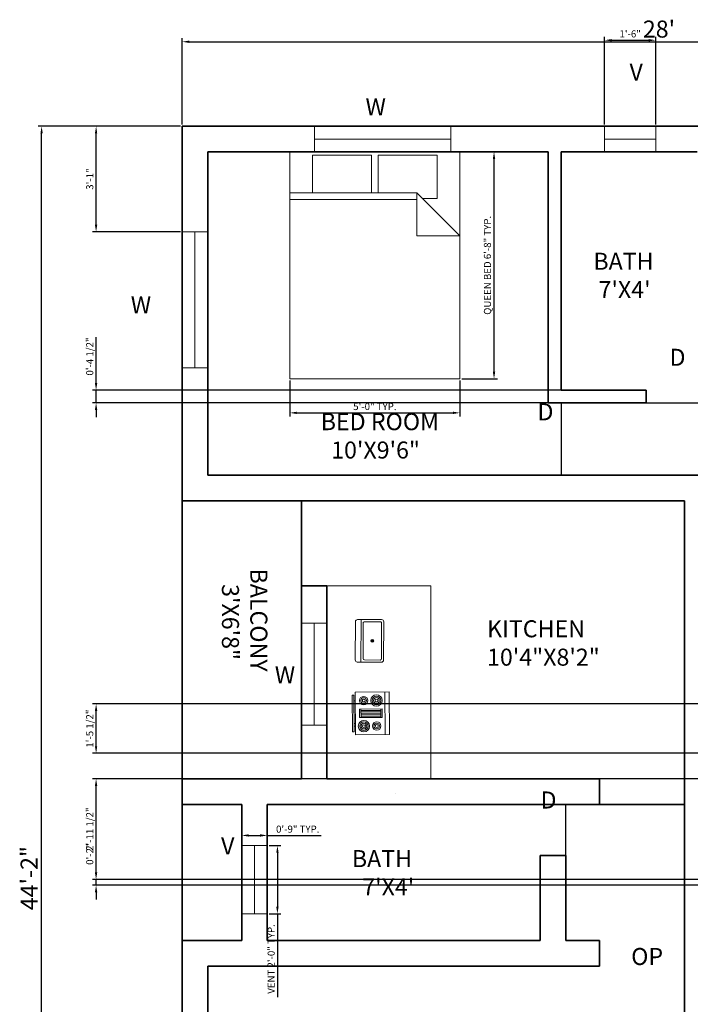
# Model space of a CAD drawing. Units: inches. Extents: x 22580 to 27643822, y 20781 to 31007121.
# Tile 2 of 3: x 27643397 to 27643633, y 31006774 to 31007121. Entities that reach past the tile are written whole.
import ezdxf

# ---------------------------------------------------------------- set-up
doc = ezdxf.new("R2010")
doc.units = ezdxf.units.IN
for name, color, linetype, lineweight in [('A-ANNO-DIMS', 2, 'Continuous', 18), ('A-ANNO-TEXT', 7, 'Continuous', 18), ('A-AREA-IDEN', 7, 'Continuous', 25), ('A-DOOR', 3, 'Continuous', 25), ('A-EQPM', 8, 'Continuous', 18), ('A-FLOR-CASE', 8, 'Continuous', 20), ('A-FLOR-FIXT', 9, 'Continuous', 18), ('A-FURN', 8, 'Continuous', 18), ('A-GLAZ', 4, 'Continuous', 18), ('A-REFR', 8, 'Continuous', 13), ('A-WALL', 7, 'Continuous', 35)]:
    doc.layers.add(name, color=color, linetype=linetype, lineweight=lineweight)
doc.styles.get("Standard").update_dxf_attribs({"font": 'arial.ttf'})
doc.dimstyles.new('ISO-25', dxfattribs={"dimtxt": 2.5, "dimasz": 2.5, "dimexe": 1.25, "dimexo": 0.625, "dimtad": 1, "dimdec": 1, "dimlunit": 3, "dimtxsty": 'Standard', "dimcen": 2.5, "dimadec": 0, "dimazin": 0, "dimtfac": 1, "dimtdec": 1, "dimtmove": 0, "dimatfit": 3, "dimfxl": 1, "dimarcsym": 0})

# ---------------------------------------------------------------- blocks, each defined once
blk = doc.blocks.new('Range-Oven - 30 in top')
for p, q in [((0, -3), (30, -3)), ((12, -6), (18, -6)), ((13, -20), (13, -6)), ((14, -6), (14, -20)), ((15, -20), (15, -6)), ((16, -6), (16, -20)), ((17, -20), (17, -6)), ((18, -20), (12, -20)), ((6, -24), (6, -25)), ((8, -25), (8, -24)), ((22, -25), (22, -24)), ((24, -24), (24, -25))]:
    blk.add_line(p, q)
for points in [[(0, -24), (0, 0), (30, 0), (30, -24)], [(12, -21), (12, -5), (18, -5), (18, -21)], [(2, -26), (2, -25), (28, -25), (28, -26)]]:
    blk.add_lwpolyline(points, close=True)
for centre, radius in [((6, -9), 4), ((6, -9), 3), ((24, -9), 3), ((6, -9), 2), ((6, -9), 1), ((24, -9), 2), ((24, -9), 1), ((6, -18), 3), ((6, -18), 2), ((6, -18), 1), ((24, -18), 4), ((24, -18), 3), ((24, -18), 2), ((24, -18), 1)]:
    blk.add_circle(centre, radius)
blk = doc.blocks.new('Bed - Queen')
for p, q in [((0, -80.00003), (0, 0)), ((0, 0), (59.99999, 0)), ((59.99999, 0), (59.99999, -80.00003)), ((7.99999, -1.2), (28.79998, -1.2)), ((7.99999, -14.4), (7.99999, -1.2)), ((28.79998, -1.2), (28.79998, -14.4)), ((31.19999, -1.2), (51.99999, -1.2)), ((31.19999, -14.4), (31.19999, -1.2)), ((51.99999, -1.2), (51.99999, -16.4)), ((0, -14.4), (44.8, -14.4)), ((44.8, -16.8), (0, -16.8)), ((59.99999, -29.6), (44.8, -14.4)), ((44.8, -14.4), (44.8, -29.6)), ((51.99999, -16.4), (46.79936, -16.4)), ((44.8, -29.6), (59.99999, -29.6)), ((59.99999, -80.00003), (0, -80.00003))]:
    blk.add_line(p, q)
blk = doc.blocks.new('Sink-single - 30 in top')
blk.add_line((-15, -3.999996), (15, -3.999996))
for points in [[(-13.5, 0), (13.5, 0)], [(-15, -18.499996), (-15, -1.5)], [(-13.5, -17.499996), (-13.5, -6.499996)], [(-12.5, -5.499996), (12.5, -5.499996)], [(13.5, -6.499996), (13.5, -17.499996)], [(15, -1.5), (15, -18.499996)], [(13.5, -19.999996), (-13.5, -19.999996)], [(12.5, -18.499996), (-12.5, -18.499996)]]:
    blk.add_lwpolyline(points)
for radius in [1, 0.5]:
    blk.add_circle((0, -11.999996), radius)
for centre, radius, start, end in [((-13.5, -1.5), 1.5, 90, 180), ((-12.5, -6.499996), 1, 90, 180), ((12.5, -6.499996), 1, 0, 90), ((13.5, -1.5), 1.5, 0, 90), ((-13.5, -18.499996), 1.5, 180, 270), ((-12.5, -17.499996), 1, 180, 270), ((12.5, -17.499996), 1, 270, 0), ((13.5, -18.499996), 1.5, 270, 0)]:
    blk.add_arc(centre, radius, start, end)
blk = doc.blocks.new('*D9')
at = {"layer": 'A-ANNO-DIMS', "color": 0, "lineweight": -2, "transparency": 16777216}
for p, q in [((27643453.96, 31007084.46), (27643453.96, 31007114.89)), ((27643456.46, 31007113.64), (27643787.46, 31007113.64)), ((27643789.96, 31007084.46), (27643789.96, 31007114.89))]:
    blk.add_line(p, q, dxfattribs=at)
at = {"layer": 'A-ANNO-DIMS', "color": 0, "transparency": 16777216}
for points in [[(27643456.46, 31007114.06), (27643456.46, 31007113.22), (27643453.96, 31007113.64)], [(27643787.46, 31007114.06), (27643787.46, 31007113.22), (27643789.96, 31007113.64)]]:
    blk.add_solid(points, dxfattribs=at)
at = {"layer": 'Defpoints', "color": 0, "transparency": 16777216}
for p in [(27643789.96, 31007113.64), (27643453.96, 31007083.83), (27643789.96, 31007083.83)]:
    blk.add_point(p, dxfattribs=at)
at = {"layer": 'A-ANNO-DIMS', "color": 0, "transparency": 16777216, "insert": (27643621.96, 31007117.33), "char_height": 6, "attachment_point": 5}
blk.add_mtext("28'", dxfattribs=at)
blk = doc.blocks.new('*D10')
at = {"layer": 'A-ANNO-DIMS', "color": 0, "lineweight": -2, "transparency": 16777216}
for p, q in [((27643453.33, 31007083.83), (27643403.16, 31007083.83)), ((27643404.41, 31006556.33), (27643404.41, 31007081.33)), ((27643453.33, 31006553.83), (27643403.16, 31006553.83))]:
    blk.add_line(p, q, dxfattribs=at)
at = {"layer": 'A-ANNO-DIMS', "color": 0, "transparency": 16777216}
for points in [[(27643404, 31007081.33), (27643404.83, 31007081.33), (27643404.41, 31007083.83)], [(27643404, 31006556.33), (27643404.83, 31006556.33), (27643404.41, 31006553.83)]]:
    blk.add_solid(points, dxfattribs=at)
at = {"layer": 'Defpoints', "color": 0, "transparency": 16777216}
for p in [(27643404.41, 31007083.83), (27643453.96, 31007083.83), (27643453.96, 31006553.83)]:
    blk.add_point(p, dxfattribs=at)
at = {"layer": 'A-ANNO-DIMS', "color": 0, "transparency": 16777216, "insert": (27643400.78, 31006818.83), "char_height": 6, "attachment_point": 5, "rotation": 90}
blk.add_mtext('44\'-2"', dxfattribs=at)
blk = doc.blocks.new('WIN-48IN')
for p, q in [((0, 9), (0, 0)), ((48, 9), (48, 0)), ((0, 4.5), (48, 4.5))]:
    blk.add_line(p, q)
blk = doc.blocks.new('VENT-24IN')
for p, q in [((0, 9), (0, 0)), ((24, 9), (24, 0)), ((0, 4.5), (24, 4.5))]:
    blk.add_line(p, q)
blk = doc.blocks.new('*D15')
at = {"layer": 'A-ANNO-DIMS', "color": 0, "lineweight": -2, "transparency": 16777216}
for p, q in [((27643484.54, 31006830.28), (27643488.76, 31006830.28)), ((27643487.51, 31006827.78), (27643487.51, 31006808.78)), ((27643484.54, 31006806.28), (27643488.76, 31006806.28)), ((27643487.51, 31006806.28), (27643487.51, 31006776.88))]:
    blk.add_line(p, q, dxfattribs=at)
at = {"layer": 'A-ANNO-DIMS', "color": 0, "transparency": 16777216}
for points in [[(27643487.09, 31006827.78), (27643487.93, 31006827.78), (27643487.51, 31006830.28)], [(27643487.09, 31006808.78), (27643487.93, 31006808.78), (27643487.51, 31006806.28)]]:
    blk.add_solid(points, dxfattribs=at)
at = {"layer": 'Defpoints', "color": 0, "transparency": 16777216}
for p in [(27643483.91, 31006830.28), (27643483.91, 31006806.28), (27643487.51, 31006806.28)]:
    blk.add_point(p, dxfattribs=at)
at = {"layer": 'A-ANNO-DIMS', "color": 0, "transparency": 16777216, "insert": (27643485.61, 31006790.33), "char_height": 2.5, "attachment_point": 5, "rotation": 90}
blk.add_mtext('VENT 2\'-0" TYP.', dxfattribs=at)
blk = doc.blocks.new('*D16')
at = {"layer": 'A-ANNO-DIMS', "color": 0, "lineweight": -2, "transparency": 16777216}
for p, q in [((27643474.91, 31006830.9), (27643474.91, 31006835.13)), ((27643483.91, 31006830.9), (27643483.91, 31006835.13)), ((27643477.41, 31006833.88), (27643481.41, 31006833.88)), ((27643483.91, 31006833.88), (27643502.9, 31006833.88))]:
    blk.add_line(p, q, dxfattribs=at)
at = {"layer": 'A-ANNO-DIMS', "color": 0, "transparency": 16777216}
for points in [[(27643477.41, 31006834.3), (27643477.41, 31006833.46), (27643474.91, 31006833.88)], [(27643481.41, 31006834.3), (27643481.41, 31006833.46), (27643483.91, 31006833.88)]]:
    blk.add_solid(points, dxfattribs=at)
at = {"layer": 'Defpoints', "color": 0, "transparency": 16777216}
for p in [(27643483.91, 31006833.88), (27643474.91, 31006830.28), (27643483.91, 31006830.28)]:
    blk.add_point(p, dxfattribs=at)
at = {"layer": 'A-ANNO-DIMS', "color": 0, "transparency": 16777216, "insert": (27643494.66, 31006835.78), "char_height": 2.5, "attachment_point": 5}
blk.add_mtext('0\'-9" TYP.', dxfattribs=at)
blk = doc.blocks.new('*D17')
at = {"layer": 'A-ANNO-DIMS', "color": 0, "lineweight": -2, "transparency": 16777216}
for p, q in [((27643552.46, 31007074.83), (27643565.09, 31007074.83)), ((27643563.84, 31006997.33), (27643563.84, 31007072.33)), ((27643552.46, 31006994.83), (27643565.09, 31006994.83))]:
    blk.add_line(p, q, dxfattribs=at)
at = {"layer": 'A-ANNO-DIMS', "color": 0, "transparency": 16777216}
for points in [[(27643563.42, 31007072.33), (27643564.25, 31007072.33), (27643563.84, 31007074.83)], [(27643563.42, 31006997.33), (27643564.25, 31006997.33), (27643563.84, 31006994.83)]]:
    blk.add_solid(points, dxfattribs=at)
at = {"layer": 'Defpoints', "color": 0, "transparency": 16777216}
for p in [(27643551.84, 31007074.83), (27643563.84, 31007074.83), (27643551.84, 31006994.83)]:
    blk.add_point(p, dxfattribs=at)
at = {"layer": 'A-ANNO-DIMS', "color": 0, "transparency": 16777216, "insert": (27643561.84, 31007034.83), "char_height": 2.5, "attachment_point": 5, "rotation": 90}
blk.add_mtext('QUEEN BED 6\'-8" TYP.', dxfattribs=at)
blk = doc.blocks.new('*D18')
at = {"layer": 'A-ANNO-DIMS', "color": 0, "lineweight": -2, "transparency": 16777216}
for p, q in [((27643491.84, 31006994.21), (27643491.84, 31006981.58)), ((27643551.84, 31006994.21), (27643551.84, 31006981.58)), ((27643494.34, 31006982.83), (27643549.34, 31006982.83))]:
    blk.add_line(p, q, dxfattribs=at)
at = {"layer": 'A-ANNO-DIMS', "color": 0, "transparency": 16777216}
for points in [[(27643494.34, 31006983.25), (27643494.34, 31006982.42), (27643491.84, 31006982.83)], [(27643549.34, 31006983.25), (27643549.34, 31006982.42), (27643551.84, 31006982.83)]]:
    blk.add_solid(points, dxfattribs=at)
at = {"layer": 'Defpoints', "color": 0, "transparency": 16777216}
for p in [(27643491.84, 31006994.83), (27643551.84, 31006994.83), (27643551.84, 31006982.83)]:
    blk.add_point(p, dxfattribs=at)
at = {"layer": 'A-ANNO-DIMS', "color": 0, "transparency": 16777216, "insert": (27643521.84, 31006984.74), "char_height": 2.5, "attachment_point": 5}
blk.add_mtext('5\'-0" TYP.', dxfattribs=at)
blk = doc.blocks.new('*D39')
at = {"layer": 'A-ANNO-DIMS', "color": 0, "lineweight": -2, "transparency": 16777216}
for p, q in [((27643661.33, 31006853.83), (27643422.36, 31006853.83)), ((27643423.61, 31006820.83), (27643423.61, 31006851.33)), ((27643661.33, 31006818.33), (27643422.36, 31006818.33))]:
    blk.add_line(p, q, dxfattribs=at)
at = {"layer": 'A-ANNO-DIMS', "color": 0, "transparency": 16777216}
for points in [[(27643423.19, 31006851.33), (27643424.02, 31006851.33), (27643423.61, 31006853.83)], [(27643423.19, 31006820.83), (27643424.02, 31006820.83), (27643423.61, 31006818.33)]]:
    blk.add_solid(points, dxfattribs=at)
at = {"layer": 'Defpoints', "color": 0, "transparency": 16777216}
for p in [(27643423.61, 31006853.83), (27643661.96, 31006853.83), (27643661.96, 31006818.33)]:
    blk.add_point(p, dxfattribs=at)
at = {"layer": 'A-ANNO-DIMS', "color": 0, "transparency": 16777216, "insert": (27643421.69, 31006836.08), "char_height": 2.5, "attachment_point": 5, "rotation": 90}
blk.add_mtext('2\'-11 1/2"', dxfattribs=at)
blk = doc.blocks.new('*D40')
at = {"layer": 'A-ANNO-DIMS', "color": 0, "lineweight": -2, "transparency": 16777216}
for p, q in [((27643423.61, 31006820.83), (27643423.61, 31006831.23)), ((27643661.33, 31006818.33), (27643422.36, 31006818.33)), ((27643423.61, 31006816.33), (27643423.61, 31006818.33)), ((27643661.33, 31006816.33), (27643422.36, 31006816.33)), ((27643423.61, 31006813.83), (27643423.61, 31006811.33))]:
    blk.add_line(p, q, dxfattribs=at)
at = {"layer": 'A-ANNO-DIMS', "color": 0, "transparency": 16777216}
for points in [[(27643423.19, 31006820.83), (27643424.02, 31006820.83), (27643423.61, 31006818.33)], [(27643423.19, 31006813.83), (27643424.02, 31006813.83), (27643423.61, 31006816.33)]]:
    blk.add_solid(points, dxfattribs=at)
at = {"layer": 'Defpoints', "color": 0, "transparency": 16777216}
for p in [(27643423.61, 31006818.33), (27643661.96, 31006818.33), (27643661.96, 31006816.33)]:
    blk.add_point(p, dxfattribs=at)
at = {"layer": 'A-ANNO-DIMS', "color": 0, "transparency": 16777216, "insert": (27643421.71, 31006827.28), "char_height": 2.5, "attachment_point": 5, "rotation": 90}
blk.add_mtext('0\'-2"', dxfattribs=at)
blk = doc.blocks.new('*D43')
at = {"layer": 'A-ANNO-DIMS', "color": 0, "lineweight": -2, "transparency": 16777216}
for p, q in [((27643670.33, 31006880.22), (27643422.36, 31006880.22)), ((27643423.61, 31006865.33), (27643423.61, 31006877.72)), ((27643670.33, 31006862.83), (27643422.36, 31006862.83))]:
    blk.add_line(p, q, dxfattribs=at)
at = {"layer": 'A-ANNO-DIMS', "color": 0, "transparency": 16777216}
for points in [[(27643423.19, 31006877.72), (27643424.02, 31006877.72), (27643423.61, 31006880.22)], [(27643423.19, 31006865.33), (27643424.02, 31006865.33), (27643423.61, 31006862.83)]]:
    blk.add_solid(points, dxfattribs=at)
at = {"layer": 'Defpoints', "color": 0, "transparency": 16777216}
for p in [(27643423.61, 31006880.22), (27643670.96, 31006880.22), (27643670.96, 31006862.83)]:
    blk.add_point(p, dxfattribs=at)
at = {"layer": 'A-ANNO-DIMS', "color": 0, "transparency": 16777216, "insert": (27643421.69, 31006871.53), "char_height": 2.5, "attachment_point": 5, "rotation": 90}
blk.add_mtext('1\'-5 1/2"', dxfattribs=at)
blk = doc.blocks.new('*D49')
at = {"layer": 'A-ANNO-DIMS', "color": 0, "lineweight": -2, "transparency": 16777216}
for p, q in [((27643602.81, 31007084.46), (27643602.81, 31007115.43)), ((27643620.81, 31007084.46), (27643620.81, 31007115.43)), ((27643605.31, 31007114.18), (27643618.31, 31007114.18))]:
    blk.add_line(p, q, dxfattribs=at)
at = {"layer": 'A-ANNO-DIMS', "color": 0, "transparency": 16777216}
for points in [[(27643605.31, 31007114.6), (27643605.31, 31007113.77), (27643602.81, 31007114.18)], [(27643618.31, 31007114.6), (27643618.31, 31007113.77), (27643620.81, 31007114.18)]]:
    blk.add_solid(points, dxfattribs=at)
at = {"layer": 'Defpoints', "color": 0, "transparency": 16777216}
for p in [(27643620.81, 31007114.18), (27643602.81, 31007083.83), (27643620.81, 31007083.83)]:
    blk.add_point(p, dxfattribs=at)
at = {"layer": 'A-ANNO-DIMS', "color": 0, "transparency": 16777216, "insert": (27643611.81, 31007116.09), "char_height": 2.5, "attachment_point": 5}
blk.add_mtext('1\'-6"', dxfattribs=at)
blk = doc.blocks.new('*D50')
at = {"layer": 'A-ANNO-DIMS', "color": 0, "lineweight": -2, "transparency": 16777216}
for p, q in [((27643453.33, 31007083.83), (27643422.36, 31007083.83)), ((27643423.61, 31007049.15), (27643423.61, 31007081.33)), ((27643453.33, 31007046.65), (27643422.36, 31007046.65))]:
    blk.add_line(p, q, dxfattribs=at)
at = {"layer": 'A-ANNO-DIMS', "color": 0, "transparency": 16777216}
for points in [[(27643423.19, 31007081.33), (27643424.02, 31007081.33), (27643423.61, 31007083.83)], [(27643423.19, 31007049.15), (27643424.02, 31007049.15), (27643423.61, 31007046.65)]]:
    blk.add_solid(points, dxfattribs=at)
at = {"layer": 'Defpoints', "color": 0, "transparency": 16777216}
for p in [(27643423.61, 31007083.83), (27643453.96, 31007083.83), (27643453.96, 31007046.65)]:
    blk.add_point(p, dxfattribs=at)
at = {"layer": 'A-ANNO-DIMS', "color": 0, "transparency": 16777216, "insert": (27643421.7, 31007065.24), "char_height": 2.5, "attachment_point": 5, "rotation": 90}
blk.add_mtext('3\'-1"', dxfattribs=at)
blk = doc.blocks.new('*D51')
at = {"layer": 'A-ANNO-DIMS', "color": 0, "lineweight": -2, "transparency": 16777216}
for p, q in [((27643423.61, 31006993.33), (27643423.61, 31007009.55)), ((27643616.83, 31006990.83), (27643422.36, 31006990.83)), ((27643423.61, 31006986.33), (27643423.61, 31006990.83)), ((27643616.83, 31006986.33), (27643422.36, 31006986.33)), ((27643423.61, 31006983.83), (27643423.61, 31006981.33))]:
    blk.add_line(p, q, dxfattribs=at)
at = {"layer": 'A-ANNO-DIMS', "color": 0, "transparency": 16777216}
for points in [[(27643423.19, 31006993.33), (27643424.02, 31006993.33), (27643423.61, 31006990.83)], [(27643423.19, 31006983.83), (27643424.02, 31006983.83), (27643423.61, 31006986.33)]]:
    blk.add_solid(points, dxfattribs=at)
at = {"layer": 'Defpoints', "color": 0, "transparency": 16777216}
for p in [(27643423.61, 31006990.83), (27643617.46, 31006990.83), (27643617.46, 31006986.33)]:
    blk.add_point(p, dxfattribs=at)
at = {"layer": 'A-ANNO-DIMS', "color": 0, "transparency": 16777216, "insert": (27643421.69, 31007002.69), "char_height": 2.5, "attachment_point": 5, "rotation": 90}
blk.add_mtext('0\'-4 1/2"', dxfattribs=at)

msp = doc.modelspace()

# ---------------------------------------------------------------- linework, layer by layer
at = {"layer": 'A-DOOR'}
for p, q in [((27643587.46, 31006986.33), (27643587.46, 31006960.83)), ((27643617.46, 31006986.33), (27643637.71, 31006986.33)), ((27643589.12, 31006826.83), (27643589.12, 31006844.83))]:
    msp.add_line(p, q, dxfattribs=at)
at = {"layer": 'A-FLOR-CASE'}
for p, q in [((27643504.96, 31006921.83), (27643541.56, 31006921.83)), ((27643541.56, 31006921.83), (27643541.56, 31006853.83))]:
    msp.add_line(p, q, dxfattribs=at)
at = {"layer": 'A-GLAZ'}
for p, q in [((27643602.81, 31007083.83), (27643602.81, 31007074.83)), ((27643620.81, 31007083.83), (27643620.81, 31007074.83)), ((27643620.81, 31007079.33), (27643602.81, 31007079.33)), ((27643495.96, 31006908.69), (27643504.96, 31006908.69)), ((27643500.46, 31006872.69), (27643500.46, 31006908.69)), ((27643495.96, 31006872.69), (27643504.96, 31006872.69))]:
    msp.add_line(p, q, dxfattribs=at)
at = {"layer": 'A-REFR'}
msp.add_line((27643528.96, 31006848.69), (27643528.96, 31006848.69), dxfattribs=at)
at = {"layer": 'A-WALL'}
for p, q in [((27643453.96, 31007083.83), (27643789.96, 31007083.83)), ((27643453.96, 31006553.83), (27643453.96, 31007083.83)), ((27643462.96, 31007074.83), (27643582.96, 31007074.83)), ((27643462.96, 31006960.83), (27643462.96, 31007074.83)), ((27643582.96, 31006986.33), (27643582.96, 31007074.83)), ((27643587.46, 31006990.83), (27643587.46, 31007074.83)), ((27643587.46, 31007074.83), (27643635.46, 31007074.83)), ((27643587.46, 31006990.83), (27643617.46, 31006990.83)), ((27643617.46, 31006986.33), (27643617.46, 31006990.83)), ((27643582.96, 31006986.33), (27643617.46, 31006986.33)), ((27643462.96, 31006960.83), (27643639.96, 31006960.83)), ((27643453.96, 31006951.83), (27643630.96, 31006951.83)), ((27643495.96, 31006853.83), (27643495.96, 31006951.83)), ((27643630.96, 31006748.84), (27643630.96, 31006951.83)), ((27643495.96, 31006921.83), (27643504.96, 31006921.83)), ((27643504.96, 31006853.83), (27643504.96, 31006921.83)), ((27643453.96, 31006853.83), (27643495.96, 31006853.83)), ((27643504.96, 31006853.83), (27643600.96, 31006853.83)), ((27643600.96, 31006844.83), (27643600.96, 31006853.83)), ((27643453.96, 31006844.83), (27643474.91, 31006844.83)), ((27643474.91, 31006844.83), (27643474.91, 31006796.83)), ((27643483.91, 31006844.83), (27643483.91, 31006796.83)), ((27643483.91, 31006844.83), (27643630.96, 31006844.83)), ((27643580.12, 31006826.83), (27643589.12, 31006826.83)), ((27643580.12, 31006796.83), (27643580.12, 31006826.83)), ((27643589.12, 31006796.83), (27643589.12, 31006826.83)), ((27643580.12, 31006805.28), (27643580.12, 31006796.83)), ((27643453.96, 31006796.83), (27643474.91, 31006796.83)), ((27643483.91, 31006796.83), (27643580.12, 31006796.83)), ((27643589.12, 31006796.83), (27643600.96, 31006796.83)), ((27643600.96, 31006796.83), (27643600.96, 31006787.83)), ((27643462.96, 31006787.83), (27643600.96, 31006787.83)), ((27643462.96, 31006679.83), (27643462.96, 31006787.83))]:
    msp.add_line(p, q, dxfattribs=at)

# ---------------------------------------------------------------- block references
at = {"layer": 'A-EQPM', "xscale": 0.5, "yscale": 0.5, "zscale": 0.5, "rotation": 270.5896289391367}
msp.add_blockref('Range-Oven - 30 in top', (27643526.87, 31006884.5), dxfattribs=at)
at = {"layer": 'A-FLOR-FIXT', "xscale": 0.5, "yscale": 0.5, "rotation": 89.74023070971818}
msp.add_blockref('Sink-single - 30 in top', (27643514.95, 31006902.49), dxfattribs=at)
at = {"layer": 'A-FURN'}
msp.add_blockref('Bed - Queen', (27643491.84, 31007074.83), dxfattribs=at)
at = {"layer": 'A-GLAZ'}
msp.add_blockref('WIN-48IN', (27643500.6, 31007074.83), dxfattribs=at)
for name, p, rotation in [('WIN-48IN', (27643462.96, 31006998.65), 90.00000003758751), ('VENT-24IN', (27643474.91, 31006830.28), 270.0000000214418)]:
    msp.add_blockref(name, p, dxfattribs=dict(at, rotation=rotation))

# ---------------------------------------------------------------- texts
at = {"layer": 'A-ANNO-TEXT', "char_height": 6, "attachment_point": 1}
for s, insert in [(' V', (27643611.58, 31007105.97)), ('W', (27643518.55, 31007093.71)), ('W', (27643435.82, 31007023.92)), (' D', (27643625.69, 31007005.41)), (' D', (27643579.15, 31006986.2)), ('W', (27643486.58, 31006893.53)), (' D', (27643580.22, 31006849.37)), (' V', (27643467.65, 31006833.19)), ('OP', (27643612.17, 31006794.21))]:
    msp.add_mtext_dynamic_manual_height_columns(s, width=6.2882, gutter_width=12.5, heights=[0], dxfattribs=dict(at, insert=insert))
at = {"layer": 'A-AREA-IDEN', "char_height": 6, "attachment_point": 1}
for s, insert in [("  BATH\\P   7'X4'", (27643595.18, 31007039.27)), ('   BED ROOM\\P     10\'X9\'6"', (27643497.27, 31006982.73)), ('    KITCHEN\\P    10\'4"X8\'2"', (27643554.04, 31006909.72)), ("    BATH\\P      7'X4'", (27643506.4, 31006828.71))]:
    msp.add_mtext_dynamic_manual_height_columns(s, width=74.9161, gutter_width=12.5, heights=[23.22], dxfattribs=dict(at, insert=insert))
at = {"layer": 'A-AREA-IDEN', "insert": (27643483.96, 31006935.3), "char_height": 6, "attachment_point": 1, "rotation": 270}
msp.add_mtext_dynamic_manual_height_columns('    BALCONY\\P       3\'X6\'8"', width=74.9161, gutter_width=12.5, heights=[23.22], dxfattribs=at)

# ---------------------------------------------------------------- dimensions: what is measured, and where the dimension line sits
at = {"layer": 'A-ANNO-DIMS'}
for base, p1, p2, override, picture, middle in [((27643789.96, 31007113.64), (27643453.96, 31007083.83), (27643789.96, 31007083.83), {"dimtxt": 6, "dimclrd": 0, "dimclre": 0, "dimclrt": 0}, '*D9', (27643621.96, 31007117.33)), ((27643620.81, 31007114.18), (27643602.81, 31007083.83), (27643620.81, 31007083.83), {"dimdec": 1, "dimlfac": 1, "dimrnd": 0, "dimzin": 1, "dimdsep": 46, "dimlunit": 4, "dimfrac": 2}, '*D49', (27643611.81, 31007116.09))]:
    dim = msp.add_linear_dim(base=base, p1=p1, p2=p2, dimstyle='ISO-25', override=override, dxfattribs=at)
    dim.commit()
    dim.dimension.update_dxf_attribs({"geometry": picture, "text_midpoint": middle})
for base, p1, p2, override, picture, middle in [((27643404.41, 31007083.83), (27643453.96, 31006553.83), (27643453.96, 31007083.83), {"dimtxt": 6, "dimclrd": 0, "dimclre": 0, "dimclrt": 0}, '*D10', (27643400.78, 31006818.83)), ((27643423.61, 31007083.83), (27643453.96, 31007046.65), (27643453.96, 31007083.83), {"dimdec": 1, "dimlfac": 1, "dimrnd": 0, "dimzin": 1, "dimdsep": 46, "dimlunit": 4, "dimfrac": 2}, '*D50', (27643421.7, 31007065.24)), ((27643423.61, 31006990.83), (27643617.46, 31006986.33), (27643617.46, 31006990.83), {"dimdec": 1, "dimlfac": 1, "dimrnd": 0, "dimzin": 1, "dimdsep": 46, "dimlunit": 4, "dimfrac": 2}, '*D51', (27643421.69, 31007002.69)), ((27643423.61, 31006880.22), (27643670.96, 31006862.83), (27643670.96, 31006880.22), {"dimdec": 1, "dimlfac": 1, "dimrnd": 0, "dimzin": 1, "dimdsep": 46, "dimlunit": 4, "dimfrac": 2}, '*D43', (27643421.69, 31006871.53)), ((27643423.61, 31006853.83), (27643661.96, 31006818.33), (27643661.96, 31006853.83), {"dimdec": 1, "dimlfac": 1, "dimrnd": 0, "dimzin": 1, "dimdsep": 46, "dimlunit": 4, "dimfrac": 2}, '*D39', (27643421.69, 31006836.08)), ((27643423.61, 31006818.33), (27643661.96, 31006816.33), (27643661.96, 31006818.33), {"dimdec": 1, "dimlfac": 1, "dimrnd": 0, "dimzin": 1, "dimdsep": 46, "dimlunit": 4, "dimfrac": 2}, '*D40', (27643421.71, 31006827.28))]:
    dim = msp.add_linear_dim(base=base, p1=p1, p2=p2, angle=90, dimstyle='ISO-25', override=override, dxfattribs=at)
    dim.commit()
    dim.dimension.update_dxf_attribs({"geometry": picture, "text_midpoint": middle})
for base, p1, p2, angle, text, picture, middle in [((27643563.84, 31007074.83), (27643551.84, 31006994.83), (27643551.84, 31007074.83), 90, 'QUEEN BED <> TYP.', '*D17', (27643561.84, 31007034.83)), ((27643483.91, 31006833.88), (27643474.91, 31006830.28), (27643483.91, 31006830.28), 0, '<> TYP.', '*D16', (27643494.66, 31006835.78)), ((27643487.51, 31006806.28), (27643483.91, 31006830.28), (27643483.91, 31006806.28), 270, 'VENT <> TYP.', '*D15', (27643485.61, 31006790.33))]:
    dim = msp.add_linear_dim(base=base, p1=p1, p2=p2, angle=angle, text=text, dimstyle='ISO-25', override={"dimdec": 1, "dimlfac": 1, "dimrnd": 0, "dimzin": 1, "dimdsep": 46, "dimlunit": 4, "dimfrac": 2}, dxfattribs=at)
    dim.commit()
    dim.dimension.update_dxf_attribs({"geometry": picture, "text_midpoint": middle})
dim = msp.add_linear_dim(base=(27643551.84, 31006982.83), p1=(27643491.84, 31006994.83), p2=(27643551.84, 31006994.83), text='<> TYP.', dimstyle='ISO-25', override={"dimdec": 1, "dimlfac": 1, "dimrnd": 0, "dimzin": 1, "dimdsep": 46, "dimlunit": 4, "dimfrac": 2}, dxfattribs=at)
dim.commit()
dim.dimension.update_dxf_attribs({"geometry": '*D18', "text_midpoint": (27643521.84, 31006984.74)})

doc.saveas('drawing.dxf')
